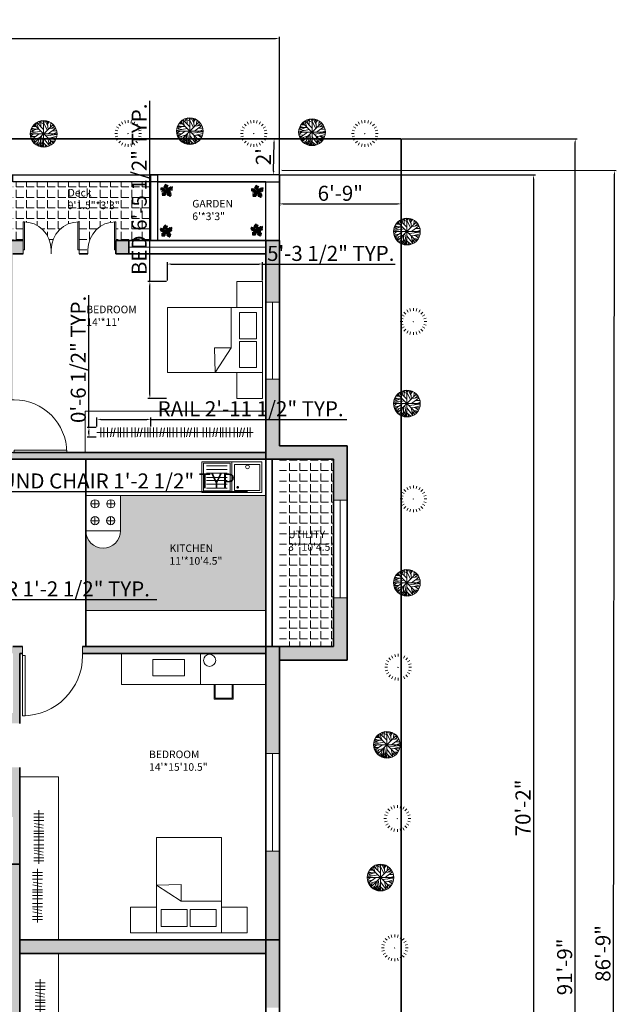
# Model space of a CAD drawing. Units: inches. Extents: x 2852 to 3654, y 1718 to 3031.
# Tile 5 of 5: x 3257 to 3654, y 2376 to 3031. Entities that reach past the tile are written whole.
import ezdxf

# ---------------------------------------------------------------- set-up
doc = ezdxf.new("R2010")
doc.units = ezdxf.units.IN
for name, color, linetype, lineweight in [('A-ANNO-DIMS', 2, 'Continuous', 18), ('A-AREA-IDEN', 7, 'Continuous', 18), ('A-DOOR', 140, 'Continuous', 18), ('A-EQPM', 210, 'Continuous', 18), ('A-FLOR-CASE', 210, 'Continuous', 18), ('A-FLOR-DECK', 52, 'Continuous', 25), ('A-FLOR-FIXT', 9, 'Continuous', 18), ('A-FLOR-PATT', 52, 'Continuous', 13), ('A-WALL-PATT', 12, 'Continuous', 13), ('C-PROP', 7, 'Continuous', 35), ('fur', 210, 'Continuous', 18), ('tree', 74, 'Continuous', 13), ('wall', 12, 'Continuous', 35), ('window', 140, 'Continuous', 18)]:
    doc.layers.add(name, color=color, linetype=linetype, lineweight=lineweight)
doc.styles.get("Standard").update_dxf_attribs({"font": 'arial.ttf'})
doc.dimstyles.new('ISO-25', dxfattribs={"dimtxt": 10, "dimasz": 2.5, "dimexe": 1.25, "dimexo": 0.625, "dimtad": 1, "dimdec": 0, "dimlunit": 4, "dimtxsty": 'Standard', "dimcen": 2.5, "dimadec": 0, "dimazin": 0, "dimtfac": 1, "dimtdec": 0, "dimtmove": 0, "dimatfit": 3, "dimfxl": 1, "dimarcsym": 0})
pattern_1 = [(0, (0, 0), (0, 6.985), [5.08, -1.905]), (90, (0, 0), (-6.985, 4e-16), [5.08, -1.905])]

# ---------------------------------------------------------------- blocks, each defined once
blk = doc.blocks.new('*U2')
for p, q in [((0, 0), (0, -6)), ((40, 0), (40, -6))]:
    blk.add_line(p, q)
blk.add_lwpolyline([(0, 0), (0, 40), (1.75, 40), (1.75, 0)], close=True)
blk.add_arc((0, 0), 40, 0, 90)
blk = doc.blocks.new('*U8')
for p, q in [((-47.498, 19.737), (-55.83, 18.344)), ((-40.615, 13.7), (-55.105, 10.913)), ((-31.5, 4.5), (-52.5, 25.5)), ((-33.37, 6.269), (-52.207, 5.34)), ((-48.585, 21.131), (-49.309, 29.026)), ((-28.299, 3.483), (-47.86, -5.805)), ((-43.513, 28.561), (-42.427, 15.558)), ((-38.442, 26.239), (-34.819, 7.663)), ((-21.416, 3.018), (-38.079, -8.128)), ((-35.544, 28.097), (-24.314, 3.947)), ((0, 0), (-31.5, 4.5)), ((-14.533, 2.09), (-30.834, 25.31)), ((-15.982, 2.09), (-30.11, -9.521)), ((-3.665, 19.273), (-27.574, 35.527)), ((-5.114, 28.097), (-24.676, 40.636)), ((-24.314, 23.917), (-2.941, 13.7)), ((0, 0), (-22.5, -19.5)), ((-7.288, 39.707), (-21.778, 46.673)), ((-6.563, 1.161), (-21.416, -8.128)), ((-20.691, 13.7), (-1.129, 4.876)), ((-8.737, 47.138), (-17.069, 52.711)), ((-10.186, 53.64), (-13.084, 55.962)), ((0, 0), (-10.5, 57)), ((-9.099, 51.782), (-6.563, 55.962)), ((-7.65, 43.423), (-2.578, 49.46)), ((-5.839, 35.992), (4.667, 48.067)), ((-5.114, 27.632), (10.463, 46.673)), ((-2.941, 16.486), (8.652, 37.85)), ((-1.129, 6.734), (9.014, 26.704)), ((0, 0), (27, 9)), ((0, 0), (18, -22.5)), ((3.942, 1.625), (11.187, 24.381)), ((6.478, 1.625), (26.04, -8.592)), ((10.101, 3.483), (17.708, 26.239)), ((11.187, 3.483), (30.749, -5.805)), ((16.259, 5.805), (23.142, 31.348)), ((18.07, 5.805), (35.096, -3.483)), ((22.055, 7.198), (27.489, 32.277)), ((24.229, 7.663), (46.688, 1.625)), ((27, 9), (48, 36)), ((27.127, 9.056), (31.112, 35.992)), ((29.662, 12.307), (48.137, 6.269)), ((31.836, 30.883), (32.561, 16.486)), ((33.285, 16.486), (48.862, 10.913)), ((35.096, 32.741), (37.27, 22.524)), ((36.183, 19.737), (48.137, 17.88)), ((38.719, 34.134), (41.979, 28.561)), ((40.53, 25.775), (48.862, 24.846)), ((43.791, 29.954), (51.036, 30.883)), ((44.153, 36.456), (45.239, 32.741)), ((-17.431, -15.094), (-42.789, -18.809)), ((-28.299, -29.026), (-42.789, -31.348)), ((-24.314, -21.596), (-42.427, -22.06)), ((-30.834, -34.135), (-42.427, -35.528)), ((-34.457, -39.708), (-40.978, -42.494)), ((-26.849, -26.24), (-40.253, -25.775)), ((-22.5, -19.5), (-37.5, -45)), ((-32.646, -36.921), (-31.921, -44.352)), ((-15.257, -12.772), (-30.11, -12.772)), ((-29.023, -30.884), (-27.936, -43.887)), ((-25.038, -23.918), (-22.865, -45.281)), ((-20.691, -18.345), (-17.793, -44.352)), ((-6.563, -5.805), (-19.967, -9.985)), ((-17.069, -15.094), (-12.721, -40.172)), ((-13.446, -11.378), (-8.737, -32.741)), ((-9.461, -8.592), (-6.201, -23.453)), ((-4.752, -3.483), (-3.665, -14.629)), ((2.493, -3.019), (-1.491, -20.202)), ((1.769, -2.555), (24.229, -9.521)), ((5.029, -6.27), (2.131, -25.775)), ((9.014, -11.378), (3.58, -35.992)), ((14.085, -16.951), (6.478, -40.172)), ((7.565, -9.056), (32.198, -14.629)), ((18.07, -22.524), (8.289, -45.745)), ((12.274, -15.094), (36.907, -18.809)), ((20.244, -30.419), (15.897, -44.816)), ((16.259, -19.738), (36.183, -22.989)), ((18, -22.5), (27, -52.5)), ((18.433, -22.524), (40.53, -29.026)), ((19.157, -25.311), (38.719, -33.206)), ((22.78, -37.85), (19.519, -48.532)), ((21.331, -32.741), (39.081, -40.636)), ((22.78, -38.314), (34.372, -44.816)), ((24.591, -45.745), (23.142, -50.854)), ((24.591, -43.423), (30.749, -47.603)), ((26.764, -49.925), (28.213, -50.854))]:
    blk.add_line(p, q)
blk = doc.blocks.new('*U9')
for p, q in [((-25.024, 42.079), (-31.077, 52.563)), ((-13.435, 46.72), (-16.606, 58.557)), ((-1.077, 60.601), (-1.077, 48.601)), ((11.28, 46.72), (14.452, 58.557)), ((22.87, 42.079), (28.923, 52.563)), ((-61.077, 0.601), (-49.077, 0.601)), ((-47.5, 13.04), (-59.033, 16.131)), ((-42.564, 24.554), (-53.039, 30.601)), ((-34.93, 34.454), (-43.503, 43.028)), ((32.776, 34.454), (41.349, 43.028)), ((40.409, 24.554), (50.884, 30.601)), ((45.346, 13.04), (56.878, 16.131)), ((58.923, 0.601), (46.923, 0.601)), ((-47.5, -11.837), (-59.033, -14.928)), ((-42.564, -23.351), (-53.039, -29.399)), ((-34.93, -33.251), (-43.503, -41.825)), ((-25.024, -40.876), (-31.077, -51.36)), ((22.87, -40.876), (28.923, -51.36)), ((32.776, -33.251), (41.349, -41.825)), ((40.409, -23.351), (50.884, -29.399)), ((45.346, -11.837), (56.878, -14.928)), ((-13.435, -45.517), (-16.606, -57.354)), ((-1.077, -59.399), (-1.077, -47.399)), ((11.28, -45.517), (14.452, -57.354))]:
    blk.add_line(p, q)
blk.add_lwpolyline([(-1.908, 0.978), (-2.67, -0.978), (0, 0)], close=True)
blk = doc.blocks.new('*U10')
for p, q in [((-40.1797, 44.558), (-36.4825, 43.2038)), ((-37.0107, 47.0408), (-35.25, 35.5298)), ((-32.6092, 50.4264), (-23.2782, 23.5674)), ((-31.2008, 51.1035), (-0.2149, 20.1818)), ((-26.4472, 46.5894), (-26.2712, 53.8116)), ((-22.0458, 42.0753), (-16.5881, 57.6486)), ((-21.1656, 55.8436), (-0.0388, 45.0094)), ((-12.5388, 54.9406), (-7.9613, 59.4546)), ((-12.3627, 32.1443), (-12.5388, 58.7776)), ((-5.3205, 59.6806), (16.5105, 16.7963)), ((2.426, 54.9406), (-1.4472, 59.9056)), ((0, 59.9996), (0, -60)), ((0.4894, 48.6208), (3.6584, 59.6806)), ((18.2711, 35.5298), (5.419, 59.6806)), ((9.8203, 51.5549), (12.8133, 58.5516)), ((19.6795, 19.5047), (16.3344, 57.6486)), ((17.0387, 51.1035), (23.2006, 55.1666)), ((17.7429, 43.6552), (25.4894, 54.2636)), ((31.6513, 50.8778), (30.2429, 30.5643)), ((31.1232, 42.5267), (35.8767, 48.1693)), ((-59.7219, 2.8025), (-12.0106, 12.0565)), ((-32.2571, 20.6333), (-59.1937, 9.348)), ((-58.6656, 12.7336), (-35.9543, 7.5424)), ((-57.081, 17.9248), (-47.0458, 14.7649)), ((-56.0247, 20.859), (-20.8134, 20.859)), ((-54.7923, 24.4702), (-47.75, 21.0847)), ((-54.6162, -24.7335), (-20.2853, 0.0941)), ((-53.2078, 27.4044), (-40.1797, 20.859)), ((-49.8627, 32.8214), (-32.7853, 32.8214)), ((-45.8134, 38.2383), (-40.5318, 33.0471)), ((-43.8768, 36.4326), (-44.405, 40.2696)), ((42, 42), (-42, -42)), ((42, -42), (-42, 42)), ((54.3626, 25.3731), (20.9119, 0.3198)), ((23.3767, 23.3417), (53.3063, 27.4044)), ((29.3626, -6.6771), (59.4682, 7.091)), ((36.2288, 25.1474), (48.9049, 35.0784)), ((37.1091, 37.1098), (46.6161, 37.5612)), ((38.5175, 13.4107), (58.2359, 13.6364)), ((-60, 0), (60, 0)), ((-59.7219, -4.8714), (-54.2641, -6.6771)), ((-45.2853, -0.1316), (-59.0177, -10.0627)), ((-58.4895, -12.3197), (-36.4825, -11.6426)), ((-57.081, -18.4138), (-45.2853, -17.9624)), ((-52.6797, -18.188), (-55.4966, -22.0251)), ((-53.2078, -27.442), (-16.7641, -16.6081)), ((-38.9472, -29.0219), (-51.4472, -30.6018)), ((-47.2219, -19.3166), (-50.2148, -26.3135)), ((-46.5177, -30.1504), (-49.5106, -33.536)), ((-32.4331, -32.4075), (-48.1021, -35.5674)), ((-43.7008, -34.6645), (-46.6937, -37.373)), ((-35.9543, -22.4765), (-44.0529, -40.5329)), ((-24.6867, -37.8244), (-38.7712, -45.7241)), ((-26.2712, -43.9185), (-34.7219, -48.6583)), ((-19.9331, -20.2194), (-28.5599, -52.721)), ((-14.6515, -36.2445), (-27.6797, -52.9467)), ((-14.8275, -15.0282), (-14.6515, -57.6865)), ((-14.6515, -32.1818), (-3.912, -59.4922)), ((-10.074, -10.0627), (-2.5036, -59.7178)), ((-6.2008, -36.2445), (17.919, -57.0094)), ((-0.0388, -19.0909), (25.8415, -53.8495)), ((9.2922, -9.1598), (59.6443, -2.8401)), ((18.6232, -18.6394), (26.7218, -53.3981)), ((18.7992, -18.6394), (57.3556, -17.2853)), ((22.8485, -36.4702), (35.3485, -48.4326)), ((26.3697, -18.4138), (58.9401, -9.8369)), ((30.419, -30.1504), (32.3556, -50.0125)), ((31.4753, -31.279), (49.6091, -33.3103)), ((38.1654, -18.188), (52.426, -29.0219)), ((41.5105, -32.6332), (46.088, -38.0501)), ((45.9119, -24.0564), (55.595, -22.2508)), ((-14.6515, -47.3041), (-25.0388, -54.3009)), ((-21.5177, -45.4984), (-19.9331, -56.1065)), ((-8.4895, -47.5298), (-11.4825, -58.5893)), ((-6.3768, -52.721), (-9.3698, -58.815)), ((8.4119, -53.1724), (3.8344, -59.4922)), ((5.9471, -46.6269), (10.5246, -58.5893)), ((24.7852, -44.8213), (23.0246, -54.978))]:
    blk.add_line(p, q)
blk.add_circle((0, 0), 60)
blk = doc.blocks.new('*D11')
at = {"layer": 'A-ANNO-DIMS', "color": 0, "lineweight": -2, "transparency": 16777216}
for p, q in [((2942.37, 2928.32), (2942.37, 3019.61)), ((2944.87, 3018.36), (3427.45, 3018.36)), ((3429.95, 2928.32), (3429.95, 3019.61))]:
    blk.add_line(p, q, dxfattribs=at)
at = {"layer": 'A-ANNO-DIMS', "color": 0, "lineweight": 100, "transparency": 16777216}
for points in [[(2944.87, 3018.78), (2944.87, 3017.95), (2942.37, 3018.36)], [(3427.45, 3018.78), (3427.45, 3017.95), (3429.95, 3018.36)]]:
    blk.add_solid(points, dxfattribs=at)
at = {"layer": 'Defpoints', "color": 0, "lineweight": 100, "transparency": 16777216}
for p in [(3429.95, 3018.36), (2942.37, 2927.69), (3429.95, 2927.69)]:
    blk.add_point(p, dxfattribs=at)
at = {"layer": 'A-ANNO-DIMS', "color": 0, "transparency": 16777216, "insert": (3186.16, 3024.09), "char_height": 10, "attachment_point": 5}
blk.add_mtext('40\'-8"', dxfattribs=at)
blk = doc.blocks.new('*D12')
at = {"layer": 'A-ANNO-DIMS', "color": 0, "lineweight": -2, "transparency": 16777216}
for p, q in [((3430.58, 2927.69), (3600.09, 2927.69)), ((3598.84, 2925.19), (3598.84, 2088.69)), ((3430.58, 2086.19), (3600.09, 2086.19))]:
    blk.add_line(p, q, dxfattribs=at)
at = {"layer": 'A-ANNO-DIMS', "color": 0, "lineweight": 100, "transparency": 16777216}
for points in [[(3598.42, 2925.19), (3599.25, 2925.19), (3598.84, 2927.69)], [(3598.42, 2088.69), (3599.25, 2088.69), (3598.84, 2086.19)]]:
    blk.add_solid(points, dxfattribs=at)
at = {"layer": 'Defpoints', "color": 0, "lineweight": 100, "transparency": 16777216}
for p in [(3429.95, 2927.69), (3429.95, 2086.19), (3598.84, 2086.19)]:
    blk.add_point(p, dxfattribs=at)
at = {"layer": 'A-ANNO-DIMS', "color": 0, "transparency": 16777216, "insert": (3593.1, 2506.94), "char_height": 10, "attachment_point": 5, "rotation": 90}
blk.add_mtext('70\'-2"', dxfattribs=at)
blk = doc.blocks.new('*D13')
at = {"layer": 'A-ANNO-DIMS', "color": 0, "lineweight": -2, "transparency": 16777216}
for p, q in [((3431.69, 2930.92), (3653.8, 2930.67)), ((3651.35, 1892.32), (3652.54, 2928.17)), ((3430.49, 1890.07), (3652.6, 1889.82))]:
    blk.add_line(p, q, dxfattribs=at)
at = {"layer": 'A-ANNO-DIMS', "color": 0, "lineweight": 100, "transparency": 16777216}
for points in [[(3652.13, 2928.17), (3652.96, 2928.17), (3652.55, 2930.67)], [(3650.94, 1892.32), (3651.77, 1892.32), (3651.35, 1889.82)]]:
    blk.add_solid(points, dxfattribs=at)
at = {"layer": 'Defpoints', "color": 0, "lineweight": 100, "transparency": 16777216}
for p in [(3431.06, 2930.92), (3652.55, 2930.67), (3429.87, 1890.07)]:
    blk.add_point(p, dxfattribs=at)
at = {"layer": 'A-ANNO-DIMS', "color": 0, "transparency": 16777216, "insert": (3646.22, 2410.25), "char_height": 10, "attachment_point": 5, "rotation": 89.93413}
blk.add_mtext('86\'-9"', dxfattribs=at)
blk = doc.blocks.new('*D14')
at = {"layer": 'A-ANNO-DIMS', "color": 0, "lineweight": -2, "transparency": 16777216}
for p, q in [((3429.95, 2927.07), (3429.95, 2907.23)), ((3510.95, 2927.07), (3510.95, 2907.23)), ((3432.45, 2908.48), (3508.45, 2908.48))]:
    blk.add_line(p, q, dxfattribs=at)
at = {"layer": 'A-ANNO-DIMS', "color": 0, "lineweight": 100, "transparency": 16777216}
for points in [[(3432.45, 2908.9), (3432.45, 2908.06), (3429.95, 2908.48)], [(3508.45, 2908.9), (3508.45, 2908.06), (3510.95, 2908.48)]]:
    blk.add_solid(points, dxfattribs=at)
at = {"layer": 'Defpoints', "color": 0, "lineweight": 100, "transparency": 16777216}
for p in [(3429.95, 2927.69), (3510.95, 2927.69), (3510.95, 2908.48)]:
    blk.add_point(p, dxfattribs=at)
at = {"layer": 'A-ANNO-DIMS', "color": 0, "transparency": 16777216, "insert": (3470.45, 2914.21), "char_height": 10, "attachment_point": 5}
blk.add_mtext('6\'-9"', dxfattribs=at)
blk = doc.blocks.new('*D15')
at = {"layer": 'A-ANNO-DIMS', "color": 0, "lineweight": -2, "transparency": 16777216}
for p, q in [((3429.33, 2951.7), (3425.2, 2951.75)), ((3426.17, 2930.24), (3426.42, 2949.24)), ((3429.01, 2927.7), (3424.89, 2927.75))]:
    blk.add_line(p, q, dxfattribs=at)
at = {"layer": 'A-ANNO-DIMS', "color": 0, "lineweight": 100, "transparency": 16777216}
for points in [[(3426, 2949.24), (3426.84, 2949.23), (3426.45, 2951.74)], [(3425.76, 2930.24), (3426.59, 2930.23), (3426.14, 2927.74)]]:
    blk.add_solid(points, dxfattribs=at)
at = {"layer": 'Defpoints', "color": 0, "lineweight": 100, "transparency": 16777216}
for p in [(3426.45, 2951.74), (3429.95, 2951.69), (3429.64, 2927.69)]:
    blk.add_point(p, dxfattribs=at)
at = {"layer": 'A-ANNO-DIMS', "color": 0, "transparency": 16777216, "insert": (3420.65, 2939.81), "char_height": 10, "attachment_point": 5, "rotation": 89.25687}
blk.add_mtext("2'", dxfattribs=at)
blk = doc.blocks.new('BED-WITH-NIGHTSTANDS')
for p, q in [((42.38, 60.42), (42.38, 33.67)), ((42.38, 33.67), (31.23, 33.67)), ((31.23, 33.67), (31.64, 17.23)), ((31.64, 17.23), (42.38, 33.67))]:
    blk.add_line(p, q)
for points in [[(63.28, 60.42), (46.24, 60.42), (46.24, 77.65), (63.28, 77.65)], [(63.28, 60.42), (0, 60.42), (0, 17.23), (63.28, 17.23)], [(59.11, 57), (47.96, 57), (47.96, 39.69), (59.11, 39.69)], [(59.11, 37.81), (47.96, 37.81), (47.96, 20.49), (59.11, 20.49)], [(63.28, 0), (46.24, 0), (46.24, 17.23), (63.28, 17.23)]]:
    blk.add_lwpolyline(points, close=True)
blk = doc.blocks.new('WARDROBE-HANGING-RAIL')
for p, q in [((0, 3.21), (35.71, 3.21)), ((2.45, 0), (2.45, 6.54)), ((4.63, 0), (4.63, 6.54)), ((6.93, 0), (6.93, 6.54)), ((8.87, 0.34), (10.08, 6.34)), ((10.83, 0.21), (12.05, 6.21)), ((14.06, 0), (14.06, 6.54)), ((15.59, 0), (15.59, 6.54)), ((17.86, 0), (17.86, 6.54)), ((20.11, 0), (20.11, 6.54)), ((23.04, 0), (23.04, 6.54)), ((25.39, 0), (25.39, 6.54)), ((26.68, 0.21), (27.9, 6.21)), ((28.71, 0.21), (29.93, 6.21)), ((31.85, 0), (31.85, 6.54)), ((33.7, 0), (33.7, 6.54))]:
    blk.add_line(p, q)
blk = doc.blocks.new('COOKTOP-4-BURNER')
for p, q in [((8.84, 29.44), (3.38, 29.44)), ((6.11, 32.18), (6.11, 26.71)), ((6.11, 26.71), (6.11, 29.44)), ((6.11, 29.44), (8.84, 29.44)), ((19.4, 29.44), (13.94, 29.44)), ((16.67, 32.18), (16.67, 26.71)), ((16.67, 26.71), (16.67, 29.44)), ((16.67, 29.44), (19.4, 29.44)), ((6.11, 20.96), (6.11, 15.5)), ((16.52, 20.96), (16.52, 15.5)), ((8.84, 18.23), (3.38, 18.23)), ((6.11, 15.5), (6.11, 18.23)), ((6.11, 18.23), (8.84, 18.23)), ((19.25, 18.23), (13.79, 18.23)), ((16.52, 15.5), (16.52, 18.23)), ((16.52, 18.23), (19.25, 18.23))]:
    blk.add_line(p, q)
blk.add_lwpolyline([(0, 35.06), (23.09, 35.06), (23.09, 11.55), (0, 11.55)], close=True)
for centre in [(6.11, 29.44), (16.67, 29.44), (6.11, 18.23), (16.52, 18.23)]:
    blk.add_circle(centre, 2.73)
blk.add_arc((11.55, 11.55), 11.55, 180, 0)
blk = doc.blocks.new('*D25')
at = {"layer": 'A-ANNO-DIMS', "color": 0, "lineweight": -2, "transparency": 16777216}
for p, q in [((3308.8, 2760.48), (3308.8, 2766.46)), ((3311.3, 2765.21), (3342.01, 2765.21)), ((3344.51, 2760.48), (3344.51, 2766.46)), ((3344.51, 2765.21), (3474.71, 2765.21))]:
    blk.add_line(p, q, dxfattribs=at)
at = {"layer": 'A-ANNO-DIMS', "color": 0, "lineweight": 100, "transparency": 16777216}
for points in [[(3311.3, 2765.62), (3311.3, 2764.79), (3308.8, 2765.21)], [(3342.01, 2765.62), (3342.01, 2764.79), (3344.51, 2765.21)]]:
    blk.add_solid(points, dxfattribs=at)
at = {"layer": 'Defpoints', "color": 0, "lineweight": 100, "transparency": 16777216}
for p in [(3344.51, 2765.21), (3308.8, 2759.85), (3344.51, 2759.85)]:
    blk.add_point(p, dxfattribs=at)
at = {"layer": 'A-ANNO-DIMS', "color": 0, "transparency": 16777216, "insert": (3410.86, 2771), "char_height": 10, "attachment_point": 5}
blk.add_mtext('RAIL 2\'-11 1/2" TYP.', dxfattribs=at)
blk = doc.blocks.new('*D26')
at = {"layer": 'A-ANNO-DIMS', "color": 0, "lineweight": -2, "transparency": 16777216}
for p, q in [((3303.45, 2759.85), (3303.45, 2847.86)), ((3308.18, 2759.85), (3302.2, 2759.85)), ((3303.45, 2755.81), (3303.45, 2757.35)), ((3308.18, 2753.31), (3302.2, 2753.31))]:
    blk.add_line(p, q, dxfattribs=at)
at = {"layer": 'A-ANNO-DIMS', "color": 0, "lineweight": 100, "transparency": 16777216}
for points in [[(3303.03, 2757.35), (3303.86, 2757.35), (3303.45, 2759.85)], [(3303.03, 2755.81), (3303.86, 2755.81), (3303.45, 2753.31)]]:
    blk.add_solid(points, dxfattribs=at)
at = {"layer": 'Defpoints', "color": 0, "lineweight": 100, "transparency": 16777216}
for p in [(3303.45, 2759.85), (3308.8, 2759.85), (3308.8, 2753.31)]:
    blk.add_point(p, dxfattribs=at)
at = {"layer": 'A-ANNO-DIMS', "color": 0, "transparency": 16777216, "insert": (3297.65, 2805.1), "char_height": 10, "attachment_point": 5, "rotation": 90}
blk.add_mtext('0\'-6 1/2" TYP.', dxfattribs=at)
blk = doc.blocks.new('*D29')
at = {"layer": 'A-ANNO-DIMS', "color": 0, "lineweight": -2, "transparency": 16777216}
for p, q in [((3204.28, 2715.63), (3204.28, 2718.45)), ((3206.78, 2717.2), (3216.43, 2717.2)), ((3218.93, 2715.63), (3218.93, 2718.45)), ((3218.93, 2717.2), (3408.86, 2717.2))]:
    blk.add_line(p, q, dxfattribs=at)
at = {"layer": 'A-ANNO-DIMS', "color": 0, "lineweight": 100, "transparency": 16777216}
for points in [[(3206.78, 2717.62), (3206.78, 2716.79), (3204.28, 2717.2)], [(3216.43, 2717.62), (3216.43, 2716.79), (3218.93, 2717.2)]]:
    blk.add_solid(points, dxfattribs=at)
at = {"layer": 'Defpoints', "color": 0, "lineweight": 100, "transparency": 16777216}
for p in [(3218.93, 2717.2), (3204.28, 2715.01), (3218.93, 2715.01)]:
    blk.add_point(p, dxfattribs=at)
at = {"layer": 'A-ANNO-DIMS', "color": 0, "transparency": 16777216, "insert": (3315.15, 2723), "char_height": 10, "attachment_point": 5}
blk.add_mtext('ROUND CHAIR 1\'-2 1/2" TYP.', dxfattribs=at)
blk = doc.blocks.new('*D31')
at = {"layer": 'A-ANNO-DIMS', "color": 0, "lineweight": -2, "transparency": 16777216}
for p, q in [((3155.23, 2647.04), (3155.23, 2644.22)), ((3157.73, 2645.47), (3167.38, 2645.47)), ((3169.88, 2647.04), (3169.88, 2644.22)), ((3169.88, 2645.47), (3348.61, 2645.47))]:
    blk.add_line(p, q, dxfattribs=at)
at = {"layer": 'A-ANNO-DIMS', "color": 0, "lineweight": 100, "transparency": 16777216}
for points in [[(3157.73, 2645.88), (3157.73, 2645.05), (3155.23, 2645.47)], [(3167.38, 2645.88), (3167.38, 2645.05), (3169.88, 2645.47)]]:
    blk.add_solid(points, dxfattribs=at)
at = {"layer": 'Defpoints', "color": 0, "lineweight": 100, "transparency": 16777216}
for p in [(3155.23, 2647.66), (3169.88, 2647.66), (3169.88, 2645.47)]:
    blk.add_point(p, dxfattribs=at)
at = {"layer": 'A-ANNO-DIMS', "color": 0, "transparency": 16777216, "insert": (3260.49, 2651.26), "char_height": 10, "attachment_point": 5}
blk.add_mtext('OPEN CHAIR 1\'-2 1/2" TYP.', dxfattribs=at)
blk = doc.blocks.new('*D33')
at = {"layer": 'A-ANNO-DIMS', "color": 0, "lineweight": -2, "transparency": 16777216}
for p, q in [((3343.92, 2856.82), (3343.92, 2976.99)), ((3354.94, 2856.82), (3342.67, 2856.82)), ((3343.92, 2781.67), (3343.92, 2854.32)), ((3354.94, 2779.17), (3342.67, 2779.17))]:
    blk.add_line(p, q, dxfattribs=at)
at = {"layer": 'A-ANNO-DIMS', "color": 0, "lineweight": 100, "transparency": 16777216}
for points in [[(3343.5, 2854.32), (3344.34, 2854.32), (3343.92, 2856.82)], [(3343.5, 2781.67), (3344.34, 2781.67), (3343.92, 2779.17)]]:
    blk.add_solid(points, dxfattribs=at)
at = {"layer": 'Defpoints', "color": 0, "lineweight": 100, "transparency": 16777216}
for p in [(3343.92, 2856.82), (3355.57, 2856.82), (3355.57, 2779.17)]:
    blk.add_point(p, dxfattribs=at)
at = {"layer": 'A-ANNO-DIMS', "color": 0, "transparency": 16777216, "insert": (3338.12, 2918.15), "char_height": 10, "attachment_point": 5, "rotation": 90}
blk.add_mtext('BED 6\'-5 1/2" TYP.', dxfattribs=at)
blk = doc.blocks.new('*D34')
at = {"layer": 'A-ANNO-DIMS', "color": 0, "lineweight": -2, "transparency": 16777216}
for p, q in [((3355.57, 2857.44), (3355.57, 2869.71)), ((3358.07, 2868.46), (3416.35, 2868.46)), ((3418.85, 2857.44), (3418.85, 2869.71)), ((3418.85, 2868.46), (3506.86, 2868.46))]:
    blk.add_line(p, q, dxfattribs=at)
at = {"layer": 'A-ANNO-DIMS', "color": 0, "lineweight": 100, "transparency": 16777216}
for points in [[(3358.07, 2868.88), (3358.07, 2868.05), (3355.57, 2868.46)], [(3416.35, 2868.88), (3416.35, 2868.05), (3418.85, 2868.46)]]:
    blk.add_solid(points, dxfattribs=at)
at = {"layer": 'Defpoints', "color": 0, "lineweight": 100, "transparency": 16777216}
for p in [(3418.85, 2868.46), (3355.57, 2856.82), (3418.85, 2856.82)]:
    blk.add_point(p, dxfattribs=at)
at = {"layer": 'A-ANNO-DIMS', "color": 0, "transparency": 16777216, "insert": (3464.11, 2874.26), "char_height": 10, "attachment_point": 5}
blk.add_mtext('5\'-3 1/2" TYP.', dxfattribs=at)
blk = doc.blocks.new('*D40')
at = {"layer": 'A-ANNO-DIMS', "color": 0, "lineweight": -2, "transparency": 16777216}
for p, q in [((3511.58, 2951.69), (3627.74, 2951.69)), ((3626.49, 1853.32), (3626.49, 2949.19)), ((3511.58, 1850.82), (3627.74, 1850.82))]:
    blk.add_line(p, q, dxfattribs=at)
at = {"layer": 'A-ANNO-DIMS', "color": 0, "lineweight": 100, "transparency": 16777216}
for points in [[(3626.07, 2949.19), (3626.9, 2949.19), (3626.49, 2951.69)], [(3626.07, 1853.32), (3626.9, 1853.32), (3626.49, 1850.82)]]:
    blk.add_solid(points, dxfattribs=at)
at = {"layer": 'Defpoints', "color": 0, "lineweight": 100, "transparency": 16777216}
for p in [(3510.95, 2951.69), (3626.49, 2951.69), (3510.95, 1850.82)]:
    blk.add_point(p, dxfattribs=at)
at = {"layer": 'A-ANNO-DIMS', "color": 0, "transparency": 16777216, "insert": (3620.76, 2401.26), "char_height": 10, "attachment_point": 5, "rotation": 90}
blk.add_mtext('91\'-9"', dxfattribs=at)

msp = doc.modelspace()

# ---------------------------------------------------------------- hatches: boundary and pattern name
at = {"layer": 'A-FLOR-PATT'}
h = msp.add_hatch(dxfattribs=at)
h.set_pattern_fill('ANGLE', color=256)
h.set_pattern_definition(pattern_1)
h.paths.add_polyline_path([(3024.95, 2923.19), (2946.87, 2923.19), (2946.87, 2884.19), (2957.35, 2884.19), (2957.35, 2896.58), (2958.16, 2896.58), (2958.16, 2896.57, -0.401453), (2975.95, 2877.98, -0.401453), (2993.74, 2896.57), (2993.74, 2896.58), (2994.55, 2896.58), (2994.55, 2877.98), (2994.55, 2875.19), (3000.35, 2875.19), (3000.35, 2877.98, -0.401453), (3018.14, 2896.57), (3018.14, 2896.58), (3018.95, 2896.58), (3018.95, 2884.19), (3024.95, 2884.19)])
h.paths.add_polyline_path([(3179.45, 2879.69), (3093.95, 2879.69), (3093.95, 2747.69), (3097.2, 2747.69), (3097.2, 2764.87), (3098.19, 2764.87), (3098.19, 2764.85, -0.401453), (3119.96, 2742.11, -0.401453), (3141.73, 2764.85), (3141.73, 2764.87), (3142.73, 2764.87), (3142.73, 2742.11), (3142.73, 2738.69), (3143.2, 2738.69), (3143.2, 2742.11, -0.401453), (3164.97, 2764.85), (3164.97, 2764.87), (3165.97, 2764.87), (3165.97, 2747.69), (3179.45, 2747.69), (3179.45, 2779.19)])
h.paths.add_polyline_path([(3344.45, 2923.19), (3252.95, 2923.19), (3252.95, 2884.19), (3259.75, 2884.19), (3259.75, 2896.58), (3260.56, 2896.58), (3260.56, 2896.57, -0.401453), (3278.35, 2877.98, -0.401453), (3296.14, 2896.57), (3296.14, 2896.58), (3296.95, 2896.58), (3296.95, 2877.98), (3296.95, 2875.19), (3302.75, 2875.19), (3302.75, 2877.98, -0.401453), (3320.54, 2896.57), (3320.54, 2896.58), (3321.35, 2896.58), (3321.35, 2884.19), (3344.45, 2884.19)])
h = msp.add_hatch(dxfattribs=at)
h.set_pattern_fill('ANGLE', color=256)
h.set_pattern_definition(pattern_1)
h.paths.add_polyline_path([(3248.45, 2849.58), (3188.45, 2849.58), (3188.45, 2844.77), (3196.45, 2844.77), (3196.45, 2842.27), (3196.95, 2842.27), (3196.95, 2844.27), (3197.95, 2844.27), (3197.95, 2841.27), (3196.45, 2841.27), (3196.45, 2838.27), (3202.45, 2840.27, -0.501317), (3221.31, 2835.31, -0.132891), (3221.31, 2833.22, -0.501323), (3202.45, 2828.27), (3196.45, 2830.27), (3196.45, 2823.77), (3188.45, 2823.77), (3188.45, 2783.69), (3215.78, 2783.69), (3215.78, 2783.73, -0.401453), (3244.71, 2813.96), (3244.71, 2813.99), (3246.03, 2813.99), (3246.03, 2783.69), (3248.45, 2783.69)])
h.paths.add_polyline_path([(3420.95, 2714.69), (3324.42, 2714.69), (3324.42, 2691.18, -1), (3301.33, 2691.18), (3301.33, 2638.19), (3420.95, 2638.19)])
h.paths.add_polyline_path([(3059.57, 2647.05, -0.132891), (3061.66, 2647.05, -0.501323), (3066.62, 2628.19), (3064.62, 2622.19), (3071.12, 2622.19), (3071.12, 2614.19), (3084.95, 2614.19), (3084.95, 2678.69), (3040.14, 2678.69), (3040.14, 2677.19), (3040.14, 2637.19), (3038.39, 2637.19), (3038.39, 2637.23, -0.401453), (3000.14, 2677.19), (3000.14, 2678.69), (2994.25, 2678.69), (2994.25, 2614.19), (3050.12, 2614.19), (3050.12, 2622.19), (3052.62, 2622.19), (3052.62, 2622.69), (3050.62, 2622.69), (3050.62, 2623.69), (3053.62, 2623.69), (3053.62, 2622.19), (3056.62, 2622.19), (3054.62, 2628.19, -0.501317)])
h.paths.add_polyline_path([(3252.95, 2533.88, -0.400409), (3223.79, 2561.89), (3223.76, 2561.89), (3223.76, 2563.17), (3252.95, 2563.17), (3252.95, 2565.48), (3192.95, 2565.48), (3192.95, 2500.92), (3252.95, 2500.92)])
h.paths.add_polyline_path([(3248.45, 2338.72), (3188.45, 2338.72), (3188.45, 2271.48), (3248.45, 2271.48), (3248.45, 2273.69)])
h.paths.add_polyline_path([(3390.34, 2273.69), (3312.95, 2273.69), (3312.95, 2224.19), (3390.34, 2224.19)])
h.paths.add_polyline_path([(3365.33, 2231.19), (3382.33, 2231.19, -0.5), (3383.33, 2230.19), (3383.33, 2226.19, -0.5), (3382.33, 2225.19), (3365.33, 2225.19, -0.5), (3364.33, 2226.19), (3364.33, 2230.19, -0.5)], flags=16)
h.paths.add_polyline_path([(3372.19, 2255.72, -0.215004), (3375.48, 2255.72, -0.48008), (3377.83, 2238.19), (3369.83, 2238.19, -0.48008)], flags=16)
h.paths.add_polyline_path([(2987.37, 2220.07), (2951.37, 2220.07), (2951.37, 2095.57), (2987.37, 2095.57)])
h = msp.add_hatch(dxfattribs=at)
h.set_pattern_fill('ANGLE', color=256)
h.set_pattern_definition(pattern_1)
h.paths.add_polyline_path([(3465.95, 2738.69), (3429.95, 2738.69), (3429.95, 2614.19), (3465.95, 2614.19)])
at = {"layer": 'A-WALL-PATT'}
h = msp.add_hatch(color=256, dxfattribs=at)
h.dxf.hatch_style = 1
h.paths.add_polyline_path([(3188.45, 2469.48), (3017.1, 2469.48), (3017.1, 2464.04), (3017.1, 2460.48), (3188.45, 2460.48)])
h.paths.add_polyline_path([(3420.95, 2614.19), (3299.24, 2614.19), (3299.24, 2609.69), (3420.95, 2609.69)])
h.paths.add_polyline_path([(3429.95, 2614.19), (3420.95, 2614.19), (3420.95, 2609.69), (3420.95, 2543.19), (3429.95, 2543.19)])
h.paths.add_polyline_path([(3474.95, 2646.58), (3465.95, 2646.58), (3465.95, 2614.19), (3429.95, 2614.19), (3429.95, 2605.19), (3474.95, 2605.19)])
h.paths.add_polyline_path([(3474.95, 2747.69), (3429.95, 2747.69), (3429.95, 2791.96), (3420.95, 2791.96), (3420.95, 2743.19), (3420.95, 2738.69), (3425.23, 2738.69), (3465.95, 2738.69), (3465.95, 2711.51), (3474.95, 2711.51)])
h.paths.add_polyline_path([(3420.95, 2743.19), (3301.03, 2743.19), (3252.95, 2743.19), (3248.45, 2743.19), (3248.45, 2738.69), (3349.1, 2738.69), (3420.95, 2738.69)])
h.paths.add_polyline_path([(3188.92, 2779.19), (3179.45, 2779.19), (3179.45, 2747.69), (3165.97, 2747.69), (3165.97, 2742.11), (3165.97, 2738.69), (3188.92, 2738.69), (3212.98, 2738.69), (3212.98, 2743.19), (3188.92, 2743.19)])
h.paths.add_polyline_path([(3093.95, 2879.69), (3093.95, 2884.19), (3089.45, 2884.19), (3084.95, 2884.19), (3084.95, 2875.19), (3084.95, 2725.28), (3089.45, 2725.28), (3089.45, 2738.69), (3097.2, 2738.69), (3097.2, 2742.11), (3097.2, 2747.69), (3093.95, 2747.69)])
h.paths.add_polyline_path([(3188.45, 2875.19), (3202.27, 2875.19), (3202.27, 2884.19), (3179.45, 2884.19), (3179.45, 2879.69), (3179.45, 2779.19), (3188.92, 2779.19), (3215.78, 2779.19), (3215.78, 2783.69), (3188.45, 2783.69)])
h.paths.add_polyline_path([(3248.45, 2884.19), (3232.5, 2884.19), (3232.5, 2875.19), (3248.45, 2875.19)])
h.paths.add_polyline_path([(3252.95, 2875.19), (3248.45, 2875.19), (3248.45, 2778.22), (3252.95, 2778.22)])
h.paths.add_polyline_path([(3252.95, 2884.19), (3248.45, 2884.19), (3248.45, 2875.19), (3252.95, 2875.19)])
h.paths.add_polyline_path([(3259.75, 2884.19), (3252.95, 2884.19), (3252.95, 2875.19), (3259.75, 2875.19), (3259.75, 2877.98)])
h.paths.add_polyline_path([(3329.96, 2884.19), (3321.35, 2884.19), (3321.35, 2877.98), (3321.35, 2875.19), (3329.96, 2875.19)])
h.paths.add_polyline_path([(3029.12, 2884.19), (3018.95, 2884.19), (3018.95, 2877.98), (3018.95, 2875.19), (3029.12, 2875.19)])
h.paths.add_polyline_path([(3429.95, 2884.19), (3420.95, 2884.19), (3420.95, 2875.19), (3420.95, 2843.21), (3429.95, 2843.21)])
h = msp.add_hatch(color=256, dxfattribs=at)
h.dxf.hatch_style = 1
h.paths.add_polyline_path([(3188.45, 2266.98), (3183.95, 2266.98), (3183.95, 2224.57), (3183.95, 2220.07), (3205.81, 2220.07), (3205.81, 2224.57), (3188.45, 2224.57)])
h.paths.add_polyline_path([(3188.45, 2367.48), (3183.95, 2367.48), (3183.95, 2266.98), (3188.45, 2266.98), (3188.45, 2271.48)])
h.paths.add_polyline_path([(3051.87, 2376.48), (3017.1, 2376.48), (3017.1, 2372.85), (3017.1, 2367.57), (3047.37, 2367.57), (3051.87, 2367.57), (3051.87, 2372.07)])
h.paths.add_polyline_path([(3197.45, 2376.48), (3197.45, 2460.48), (3225.82, 2460.48), (3225.82, 2469.48), (3188.45, 2469.48), (3188.45, 2376.48), (3051.87, 2376.48), (3051.87, 2372.07), (3051.87, 2367.48), (3197.45, 2367.48)])
h.paths.add_polyline_path([(3257.45, 2410.19), (3257.45, 2469.48), (3247.17, 2469.48), (3247.17, 2460.48), (3248.45, 2460.48), (3248.45, 2376.48), (3218.8, 2376.48), (3218.8, 2367.48), (3257.45, 2367.48)])
h.paths.add_polyline_path([(3257.45, 2367.48), (3252.95, 2367.48), (3252.95, 2278.19), (3257.45, 2278.19)])
h.paths.add_polyline_path([(3420.95, 2278.19), (3308.45, 2278.19), (3308.45, 2273.69), (3420.95, 2273.69)])
h.paths.add_polyline_path([(3257.45, 2527.51), (3257.45, 2533.88), (3252.95, 2533.88), (3252.95, 2469.48), (3257.45, 2469.48)])
h.paths.add_polyline_path([(3257.45, 2609.69), (3259.24, 2609.69), (3259.24, 2614.19), (3252.95, 2614.19), (3227.77, 2614.19), (3227.77, 2611.84), (3227.77, 2609.69), (3252.95, 2609.69), (3252.95, 2563.17), (3253.06, 2563.17), (3257.45, 2563.17)])
h.paths.add_polyline_path([(3196.43, 2614.19), (3188.45, 2614.19), (3188.45, 2569.84), (3188.45, 2469.48), (3192.95, 2469.48), (3192.95, 2565.48), (3252.95, 2565.48), (3252.95, 2569.98), (3192.95, 2569.98), (3192.95, 2609.69), (3196.43, 2609.69), (3196.43, 2611.84)])
h = msp.add_hatch(color=256, dxfattribs=at)
h.dxf.hatch_style = 1
h.paths.add_polyline_path([(3429.87, 2117.5), (3420.87, 2117.5), (3420.87, 2095.19), (3276.87, 2095.19), (3276.87, 2086.19), (3429.87, 2086.19)])
h.paths.add_polyline_path([(3429.95, 2278.19), (3420.95, 2278.19), (3420.95, 2273.69), (3420.95, 2224.19), (3429.95, 2224.19)])
h.paths.add_polyline_path([(3429.95, 2309.24), (3420.95, 2309.24), (3420.95, 2278.19), (3429.95, 2278.19)])
h.paths.add_polyline_path([(3429.95, 2419.19), (3420.95, 2419.19), (3420.95, 2410.19), (3420.95, 2374.17), (3429.95, 2374.17)])
h.paths.add_polyline_path([(3429.95, 2478.26), (3420.95, 2478.26), (3420.95, 2419.19), (3429.95, 2419.19)])
h.paths.add_polyline_path([(3420.95, 2419.19), (3257.45, 2419.19), (3257.45, 2410.19), (3283.32, 2410.19), (3420.95, 2410.19)])

# ---------------------------------------------------------------- linework, layer by layer
at = {"layer": 'A-FLOR-CASE'}
for p, q in [((3301.33, 2738.69), (3301.33, 2714.69)), ((3301.33, 2714.69), (3420.95, 2714.69)), ((3301.33, 2691.18), (3301.33, 2714.69)), ((3301.33, 2614.19), (3301.33, 2638.19)), ((3301.33, 2638.19), (3420.95, 2638.19))]:
    msp.add_line(p, q, dxfattribs=at)
for points in [[(3301.03, 2743.19), (3420.95, 2743.19), (3420.95, 2770.68), (3301.03, 2770.68)], [(3257.45, 2419.19), (3283.32, 2419.19), (3283.32, 2527.51), (3257.45, 2527.51)], [(3257.45, 2301.87), (3283.32, 2301.87), (3283.32, 2410.19), (3257.45, 2410.19)]]:
    msp.add_lwpolyline(points, close=True, dxfattribs=at)
at = {"layer": 'A-FLOR-DECK'}
for p, q in [((3248.45, 2927.69), (3344.45, 2927.69)), ((3429.95, 2927.69), (3344.45, 2927.69)), ((3344.45, 2927.69), (3344.45, 2884.19)), ((3429.95, 2884.19), (3429.95, 2927.69)), ((3420.95, 2923.19), (3252.95, 2923.19)), ((3348.95, 2923.19), (3348.95, 2884.19)), ((3420.95, 2884.19), (3420.95, 2923.19))]:
    msp.add_line(p, q, dxfattribs=at)
for points in [[(3252.95, 2927.69), (3348.95, 2927.69), (3348.95, 2923.19), (3252.95, 2923.19)], [(3344.45, 2927.69), (3348.95, 2927.69), (3348.95, 2884.19), (3344.45, 2884.19)], [(3348.95, 2923.19), (3429.95, 2923.19), (3429.95, 2927.69), (3348.95, 2927.69)]]:
    msp.add_lwpolyline(points, close=True, dxfattribs=at)
at = {"layer": 'A-FLOR-FIXT'}
for p, q in [((3398.42, 2737.07), (3398.42, 2716.61)), ((3381.47, 2734.33), (3395.32, 2734.33)), ((3381.47, 2731.94), (3395.32, 2731.94)), ((3381.47, 2729.47), (3395.32, 2729.47)), ((3381.47, 2726.68), (3395.32, 2726.68)), ((3381.47, 2724.52), (3395.32, 2724.52)), ((3381.47, 2722.05), (3395.32, 2722.05)), ((3381.47, 2719.57), (3395.32, 2719.57))]:
    msp.add_line(p, q, dxfattribs=at)
for points in [[(3418.41, 2737.07), (3378.44, 2737.07), (3378.44, 2716.61), (3418.41, 2716.61)], [(3379.62, 2736.04), (3397.33, 2736.04), (3397.33, 2717.79), (3379.62, 2717.79)], [(3400.04, 2735.34), (3417.06, 2735.34), (3417.06, 2717.95), (3400.04, 2717.95)]]:
    msp.add_lwpolyline(points, close=True, dxfattribs=at)
msp.add_circle((3408.78, 2733.64), 1.24, dxfattribs=at)
at = {"layer": 'C-PROP'}
for p, q in [((2894.37, 2951.69), (3474.95, 2951.69)), ((3474.95, 2951.69), (3510.95, 2951.69)), ((3510.95, 2951.69), (3510.95, 1890.07))]:
    msp.add_line(p, q, dxfattribs=at)
at = {"layer": 'fur'}
for p, q in [((3387.32, 2589.06), (3386.61, 2589.06)), ((3386.61, 2589.06), (3386.61, 2579.25)), ((3387.32, 2589.06), (3387.32, 2589.06)), ((3399.33, 2579.25), (3399.33, 2589.06)), ((3386.61, 2579.25), (3399.33, 2579.25))]:
    msp.add_line(p, q, dxfattribs=at)
for points in [[(3325.13, 2609.69), (3420.95, 2609.69), (3420.95, 2589.06), (3325.13, 2589.06)], [(3345.95, 2605.52), (3366.88, 2605.52), (3366.88, 2594.67), (3345.95, 2594.67)], [(3377.61, 2589.06), (3420.95, 2589.06), (3420.95, 2609.69), (3377.61, 2609.69)], [(3387.32, 2589.06), (3398.58, 2589.06), (3398.58, 2579.99), (3387.32, 2579.99)]]:
    msp.add_lwpolyline(points, close=True, dxfattribs=at)
msp.add_circle((3383.61, 2605.05), 4.03, dxfattribs=at)
at = {"layer": 'wall'}
for p, q in [((3259.75, 2884.19), (3248.45, 2884.19)), ((3429.95, 2884.19), (3321.35, 2884.19)), ((3420.95, 2875.19), (3420.95, 2884.19)), ((3429.95, 2747.69), (3429.95, 2884.19)), ((3259.75, 2875.19), (3252.95, 2875.19)), ((3302.75, 2875.19), (3296.95, 2875.19)), ((3420.95, 2875.19), (3321.35, 2875.19)), ((3420.95, 2743.19), (3420.95, 2875.19)), ((3252.95, 2743.19), (3349.1, 2743.19)), ((3420.95, 2743.19), (3288.95, 2743.19)), ((3420.95, 2738.69), (3420.95, 2743.19)), ((3474.95, 2747.69), (3429.95, 2747.69)), ((3474.95, 2605.19), (3474.95, 2747.69)), ((3248.45, 2738.69), (3349.1, 2738.69)), ((3420.95, 2738.69), (3288.95, 2738.69)), ((3301.33, 2738.69), (3301.33, 2614.19)), ((3420.95, 2614.19), (3420.95, 2738.69)), ((3465.95, 2738.69), (3420.95, 2738.69)), ((3425.23, 2614.19), (3425.23, 2738.69)), ((3465.95, 2614.19), (3465.95, 2738.69)), ((3259.24, 2614.19), (3252.95, 2614.19)), ((3429.95, 2614.19), (3299.24, 2614.19)), ((3420.95, 2609.69), (3420.95, 2614.19)), ((3429.95, 2419.19), (3429.95, 2614.19)), ((3429.95, 2614.19), (3465.95, 2614.19)), ((3259.24, 2609.69), (3257.45, 2609.69)), ((3257.45, 2563.17), (3257.45, 2609.69)), ((3420.95, 2609.69), (3299.24, 2609.69)), ((3420.95, 2419.19), (3420.95, 2609.69)), ((3429.95, 2605.19), (3474.95, 2605.19)), ((3257.45, 2469.48), (3257.45, 2533.88)), ((3257.45, 2469.48), (3188.45, 2469.48)), ((3257.45, 2367.48), (3257.45, 2469.48)), ((3429.95, 2419.19), (3257.45, 2419.19)), ((3420.95, 2410.19), (3420.95, 2419.19)), ((3429.95, 2278.19), (3429.95, 2419.19)), ((3420.95, 2410.19), (3257.45, 2410.19)), ((3420.95, 2278.19), (3420.95, 2410.19))]:
    msp.add_line(p, q, dxfattribs=at)
msp.add_lwpolyline([(3321.35, 2875.19), (3329.96, 2875.19), (3329.96, 2884.19), (3321.35, 2884.19)], close=True, dxfattribs=at)
at = {"layer": 'window'}
for p, q in [((3329.96, 2879.69), (3420.95, 2879.69)), ((3425.45, 2843.21), (3425.45, 2791.96)), ((3470.45, 2646.58), (3470.45, 2711.51)), ((3425.45, 2478.26), (3425.45, 2543.19))]:
    msp.add_line(p, q, dxfattribs=at)
for points in [[(3329.96, 2884.19), (3420.95, 2884.19), (3420.95, 2875.19), (3329.96, 2875.19)], [(3420.95, 2843.21), (3429.95, 2843.21), (3429.95, 2791.96), (3420.95, 2791.96)], [(3420.95, 2738.69), (3425.23, 2738.69), (3425.23, 2614.19), (3420.95, 2614.19)], [(3465.95, 2711.51), (3474.95, 2711.51), (3474.95, 2646.58), (3465.95, 2646.58)], [(3420.95, 2543.19), (3429.95, 2543.19), (3429.95, 2478.26), (3420.95, 2478.26)]]:
    msp.add_lwpolyline(points, close=True, dxfattribs=at)

# ---------------------------------------------------------------- block references
at = {"layer": 'A-DOOR', "yscale": 0.4650478663129195, "zscale": 0.4650478663129195}
for p, xscale in [((3259.75, 2877.98), 0.4650478663129195), ((3296.95, 2877.98), -0.4650478663129195), ((3321.35, 2877.98), -0.4650478663129195)]:
    msp.add_blockref('*U2', p, dxfattribs=dict(at, xscale=xscale))
at = {"layer": 'A-DOOR', "xscale": -0.8757866022194583, "yscale": 0.8757866022194583, "zscale": 0.8757866022194583, "rotation": 270}
msp.add_blockref('*U2', (3253.71, 2743.19), dxfattribs=at)
at = {"layer": 'A-DOOR', "xscale": -1, "rotation": 180}
msp.add_blockref('*U2', (3259.24, 2608.19), dxfattribs=at)
at = {"layer": 'A-EQPM'}
msp.add_blockref('COOKTOP-4-BURNER', (3301.33, 2679.64), dxfattribs=at)
at = {"layer": 'A-FLOR-CASE'}
for p in [(3308.8, 2753.31), (3341.65, 2753.31), (3376.84, 2753.31)]:
    msp.add_blockref('WARDROBE-HANGING-RAIL', p, dxfattribs=at)
at = {"layer": 'A-FLOR-CASE', "rotation": 270.0000000000057}
for p in [(3266.86, 2505.53), (3266, 2466.56), (3267.8, 2393.13)]:
    msp.add_blockref('WARDROBE-HANGING-RAIL', p, dxfattribs=at)
at = {"layer": 'fur'}
msp.add_blockref('BED-WITH-NIGHTSTANDS', (3355.57, 2779.16), dxfattribs=at)
at = {"layer": 'fur', "rotation": 270.0000000000026}
msp.add_blockref('BED-WITH-NIGHTSTANDS', (3331, 2487.28), dxfattribs=at)
at = {"layer": 'tree'}
for name, p, xscale, yscale, zscale in [('*U10', (3370.45, 2956.77), 0.1480989313836924, 0.1480989313836924, 0.1480989313836924), ('*U10', (3451.64, 2956.06), 0.1480989313836924, 0.1480989313836924, 0.1480989313836924), ('*U10', (3273.36, 2954.99), 0.1480989313836924, 0.1480989313836924, 0.1480989313836924), ('*U9', (3329.65, 2955.15), 0.1480989313836924, 0.1480989313836924, 0.1480989313836924), ('*U9', (3413.14, 2955.15), 0.1480989313836924, 0.1480989313836924, 0.1480989313836924), ('*U9', (3486.97, 2955.15), 0.1480989313836924, 0.1480989313836924, 0.1480989313836924), ('*U8', (3355.24, 2917.25), 0.0764996412196377, 0.0764996412196377, 0.0764996412196377), ('*U8', (3415.48, 2916.6), 0.0764996412196377, 0.0764996412196377, 0.0764996412196377), ('*U8', (3354.91, 2890.25), 0.0764996412196377, 0.0764996412196377, 0.0764996412196377), ('*U8', (3415.15, 2890.91), 0.0764996412196377, 0.0764996412196377, 0.0764996412196377), ('*U10', (3514.72, 2890.04), 0.1480989313836924, 0.1480989313836924, 0.1480989313836924), ('*U9', (3519.16, 2830.15), 0.1480989313836924, 0.1480989313836924, 0.1480989313836924), ('*U10', (3514.72, 2775.7), 0.1480989313836924, 0.1480989313836924, 0.1480989313836924), ('*U9', (3519.16, 2712.25), 0.1480989313836924, 0.1480989313836924, 0.1480989313836924), ('*U10', (3514.72, 2656.59), 0.1480989313836924, 0.1480989313836924, 0.1480989313836924), ('*U9', (3509.05, 2600.36), 0.1480989313836924, 0.1480989313836924, 0.1480989313836924), ('*U10', (3501.39, 2548.92), 0.1480989313836924, 0.1480989313836924, 0.1480989313836924), ('*U9', (3508.51, 2499.87), 0.1480989313836924, 0.1480989313836924, 0.1480989313836924), ('*U10', (3497.14, 2460.63), 0.1480989313836924, 0.1480989313836924, 0.1480989313836924), ('*U9', (3506.75, 2413.87), 0.1480989313836924, 0.1480989313836924, 0.1480989313836924)]:
    msp.add_blockref(name, p, dxfattribs=dict(at, xscale=xscale, yscale=yscale, zscale=zscale))

# ---------------------------------------------------------------- texts
at = {"layer": 'A-AREA-IDEN', "attachment_point": 1}
for s, insert, char_height in [('Deck\\P9\'1.5"*3\'3"', (3289.34, 2918.42), 5.0412), ('GARDEN\\P6\'*3\'3"', (3372.1, 2911.13), 5.041), ("BEDROOM\\P14'*11'", (3301.71, 2840.8), 5.041), ('UTILITY\\P3\'*10\'4.5"', (3435.78, 2691.32), 5.041), ('KITCHEN\\P11\'*10\'4.5"', (3356.97, 2682.08), 5.0412), ('BEDROOM\\P14\'*15\'10.5"', (3343.38, 2545.07), 5.0412)]:
    msp.add_mtext_dynamic_manual_height_columns(s, width=98.3816, gutter_width=25.21, heights=[0], dxfattribs=dict(at, insert=insert, char_height=char_height))

# ---------------------------------------------------------------- dimensions: what is measured, and where the dimension line sits
at = {"layer": 'A-ANNO-DIMS'}
for base, p1, p2, picture, middle in [((3429.95, 3018.36), (2942.37, 2927.69), (3429.95, 2927.69), '*D11', (3186.16, 3024.09)), ((3510.95, 2908.48), (3429.95, 2927.69), (3510.95, 2927.69), '*D14', (3470.45, 2914.21))]:
    dim = msp.add_linear_dim(base=base, p1=p1, p2=p2, dimstyle='ISO-25', override={"dimclrd": 0, "dimclre": 0, "dimclrt": 0}, dxfattribs=at)
    dim.commit()
    dim.dimension.update_dxf_attribs({"geometry": picture, "text_midpoint": middle})
for base, p1, p2, text, picture, middle in [((3343.9196, 2856.8166), (3355.5673, 2779.1652), (3355.5673, 2856.8166), 'BED <> TYP.', '*D33', (3338.124, 2918.151)), ((3303.45, 2759.85), (3308.8, 2753.31), (3308.8, 2759.85), '<> TYP.', '*D26', (3297.65, 2805.1))]:
    dim = msp.add_linear_dim(base=base, p1=p1, p2=p2, angle=90, text=text, dimstyle='ISO-25', override={"dimdec": 1, "dimlfac": 1, "dimrnd": 0, "dimzin": 1, "dimdsep": 46, "dimlunit": 4, "dimfrac": 2}, dxfattribs=at)
    dim.commit()
    dim.dimension.update_dxf_attribs({"geometry": picture, "text_midpoint": middle})
for p1, p2, distance, picture, middle in [((3429.64, 2927.69), (3429.95, 2951.69), 3.5, '*D15', (3420.65, 2939.81)), ((3429.87, 1890.07), (3431.06, 2930.92), -221.48, '*D13', (3646.22, 2410.25))]:
    dim = msp.add_aligned_dim(p1=p1, p2=p2, distance=distance, dimstyle='ISO-25', override={"dimclrd": 0, "dimclre": 0, "dimclrt": 0}, dxfattribs=at)
    dim.commit()
    dim.dimension.update_dxf_attribs({"geometry": picture, "text_midpoint": middle})
for base, p1, p2, override, picture, middle in [((3626.49, 2951.69), (3510.95, 1850.82), (3510.95, 2951.69), {"dimdec": 1, "dimlfac": 1, "dimrnd": 0, "dimzin": 1, "dimdsep": 46, "dimlunit": 4, "dimfrac": 2}, '*D40', (3620.76, 2401.26)), ((3598.8351856, 2086.1927699), (3429.95105595, 2927.6927699), (3429.95105595, 2086.1927699), {"dimclrd": 0, "dimclre": 0, "dimclrt": 0}, '*D12', (3593.10445572, 2506.9427699))]:
    dim = msp.add_linear_dim(base=base, p1=p1, p2=p2, angle=90, dimstyle='ISO-25', override=override, dxfattribs=at)
    dim.commit()
    dim.dimension.update_dxf_attribs({"geometry": picture, "text_midpoint": middle})
for base, p1, p2, text, picture, middle in [((3418.85, 2868.46), (3355.57, 2856.82), (3418.85, 2856.82), '<> TYP.', '*D34', (3464.11, 2874.26)), ((3344.51, 2765.21), (3308.8, 2759.85), (3344.51, 2759.85), 'RAIL <> TYP.', '*D25', (3410.86, 2771)), ((3218.9266, 2717.2021), (3204.2806, 2715.0052), (3218.9266, 2715.0052), 'ROUND CHAIR <> TYP.', '*D29', (3315.145, 2723.0011)), ((3169.8784, 2645.4653), (3155.2325, 2647.6622), (3169.8784, 2647.6622), 'OPEN CHAIR <> TYP.', '*D31', (3260.4932, 2651.2642))]:
    dim = msp.add_linear_dim(base=base, p1=p1, p2=p2, text=text, dimstyle='ISO-25', override={"dimdec": 1, "dimlfac": 1, "dimrnd": 0, "dimzin": 1, "dimdsep": 46, "dimlunit": 4, "dimfrac": 2}, dxfattribs=at)
    dim.commit()
    dim.dimension.update_dxf_attribs({"geometry": picture, "text_midpoint": middle})

doc.saveas('drawing.dxf')
